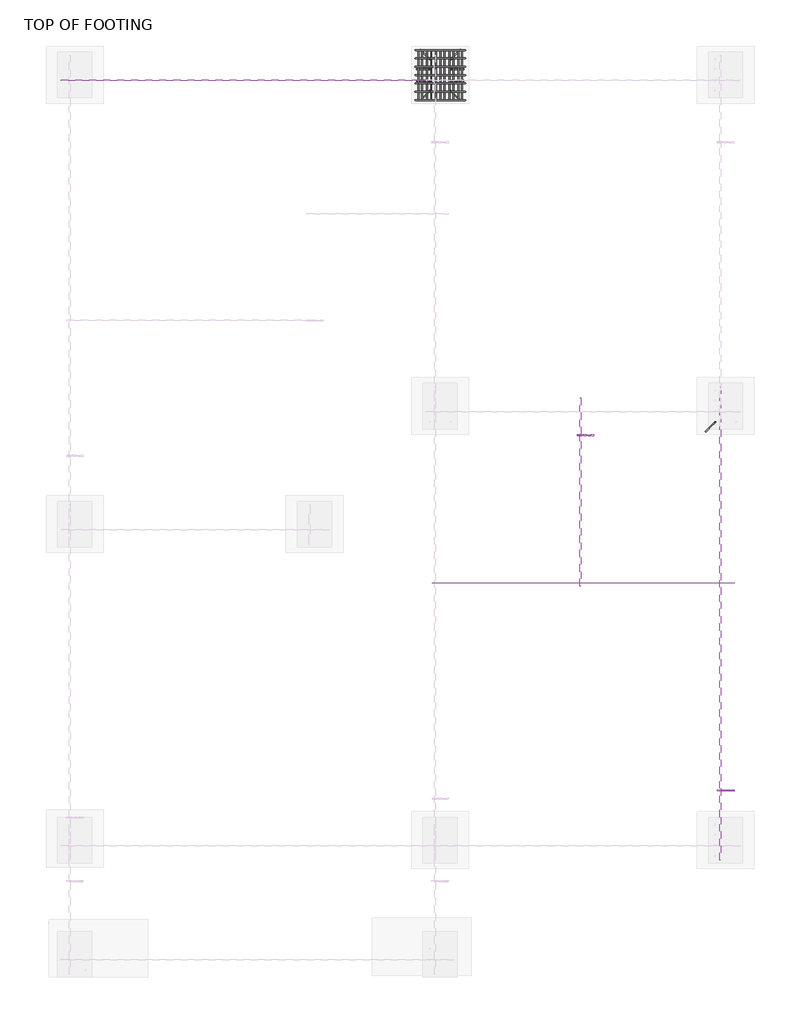
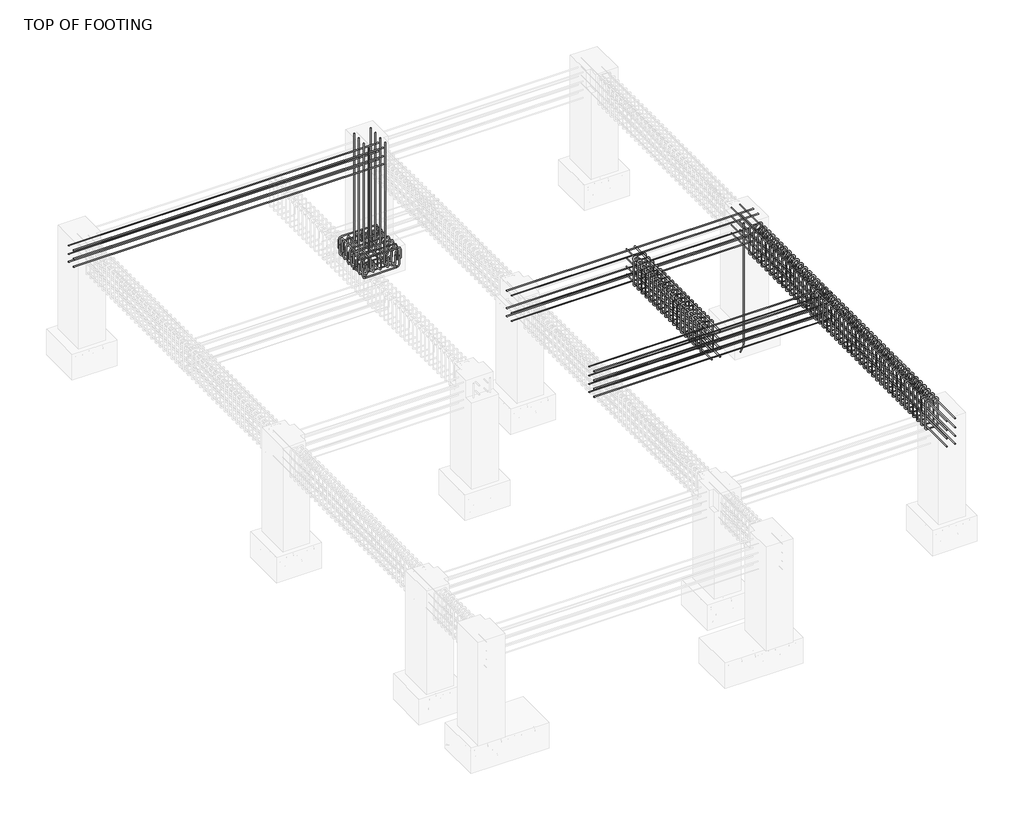
# One storey, part 7 of 8: 31 reinforcing bars.
"""IFC4 building model written with IfcOpenShell, lengths in millimetres."""

from ifc_helpers import new_model, si_unit, point, frame, origin, place, context, project, spatial, polyline, circle_curve, trimmed, segment, composite_curve, source, transform, mapped, element, save
from ifc_brep_helpers import swept_disk

model = new_model("IFC4")

# Units and contexts
model_context = context("Model", 3, world=origin())
ifc_project = project(units=[si_unit("LENGTHUNIT", "METRE", prefix="MILLI")], contexts=[model_context])

# Site, building, storey
site = spatial("IfcSite", under=ifc_project)
building = spatial("IfcBuilding", under=site)
storey = spatial("IfcBuildingStorey", under=building, Name="TOP OF FOOTING", Elevation=-1828.8)

# Reinforcing bars
placement = place(None, origin())
reinforcing_bar_shape = source(origin(), model_context, "Body", "SolidModel", [
    swept_disk(composite_curve([segment(polyline([(-1395.5877818, 9895.6420243, -2021.245224), (-1395.5877818, 9895.6420243, -2168.545224)]), True, "CONTINUOUS"), segment(trimmed(circle_curve(frame((-1441.9377818, 9895.6420243, -2168.545224), z_axis=(0.0, 1.0, 0.0), x_axis=(46.350000000000136, 0.0, 0.0)), 46.35), [point((-1395.5877818, 9895.6420243, -2168.545224))], [point((-1441.9377818, 9895.6420243, -2214.895224))], True, "CARTESIAN"), True, "CONTINUOUS"), segment(polyline([(-1441.9377818, 9895.6420243, -2214.895224), (-1962.8758647, 9895.6420243, -2214.895224)]), True, "CONTINUOUS"), segment(trimmed(circle_curve(frame((-1962.8758647, 9895.6420243, -2168.545224), z_axis=(0.0, 1.0, 0.0), x_axis=(0.0, 0.0, -46.34999999999991)), 46.35), [point((-1962.8758647, 9895.6420243, -2214.895224))], [point((-2009.2258647, 9895.6420243, -2168.545224))], True, "CARTESIAN"), True, "CONTINUOUS"), segment(polyline([(-2009.2258647, 9895.6420243, -2168.545224), (-2009.2258647, 9895.6420243, -2021.245224)]), True, "CONTINUOUS")], self_intersect=False), 6.35),
])
element("IfcReinforcingBar", 1, at=placement, inside=storey, context=model_context, shape_type="MappedRepresentation", body=[
    mapped(reinforcing_bar_shape, transform((0.0, 0.0, 0.0), x_axis=(1.0, 0.0, 0.0), y_axis=(0.0, 1.0, 0.0), z_axis=(0.0, 0.0, 1.0))),
    mapped(reinforcing_bar_shape, transform((0.0, -109.55, 0.0), x_axis=(1.0, 0.0, 0.0), y_axis=(0.0, 1.0, 0.0), z_axis=(0.0, 0.0, 1.0))),
    mapped(reinforcing_bar_shape, transform((0.0, -219.1, 0.0), x_axis=(1.0, 0.0, 0.0), y_axis=(0.0, 1.0, 0.0), z_axis=(0.0, 0.0, 1.0))),
    mapped(reinforcing_bar_shape, transform((0.0, -328.65, 0.0), x_axis=(1.0, 0.0, 0.0), y_axis=(0.0, 1.0, 0.0), z_axis=(0.0, 0.0, 1.0))),
    mapped(reinforcing_bar_shape, transform((0.0, -438.2, 0.0), x_axis=(1.0, 0.0, 0.0), y_axis=(0.0, 1.0, 0.0), z_axis=(0.0, 0.0, 1.0))),
    mapped(reinforcing_bar_shape, transform((0.0, -547.75, 0.0), x_axis=(1.0, 0.0, 0.0), y_axis=(0.0, 1.0, 0.0), z_axis=(0.0, 0.0, 1.0))),
    mapped(reinforcing_bar_shape, transform((0.0, -657.3, 0.0), x_axis=(1.0, 0.0, 0.0), y_axis=(0.0, 1.0, 0.0), z_axis=(0.0, 0.0, 1.0))),
])
reinforcing_bar_2_shape = source(origin(), model_context, "Body", "SolidModel", [
    swept_disk(composite_curve([segment(polyline([(-2031.1461367, 9895.6420243, -2068.8), (-2031.1461367, 9895.6420243, -1921.5)]), True, "CONTINUOUS"), segment(trimmed(circle_curve(frame((-1984.7961367, 9895.6420243, -1921.5), z_axis=(0.0, 1.0, 0.0), x_axis=(-46.34999999999991, 0.0, 0.0)), 46.35), [point((-2031.1461367, 9895.6420243, -1921.5))], [point((-1984.7961367, 9895.6420243, -1875.15))], True, "CARTESIAN"), True, "CONTINUOUS"), segment(polyline([(-1984.7961367, 9895.6420243, -1875.15), (-1420.1961367, 9895.6420243, -1875.15)]), True, "CONTINUOUS"), segment(trimmed(circle_curve(frame((-1420.1961367, 9895.6420243, -1921.5), z_axis=(0.0, 1.0, 0.0), x_axis=(0.0, 0.0, 46.34999999999991)), 46.35), [point((-1420.1961367, 9895.6420243, -1875.15))], [point((-1373.8461367, 9895.6420243, -1921.5))], True, "CARTESIAN"), True, "CONTINUOUS"), segment(polyline([(-1373.8461367, 9895.6420243, -1921.5), (-1373.8461367, 9895.6420243, -2068.8)]), True, "CONTINUOUS")], self_intersect=False), 6.35),
])
element("IfcReinforcingBar", 2, at=placement, inside=storey, context=model_context, shape_type="MappedRepresentation", body=[
    mapped(reinforcing_bar_2_shape, transform((0.0, 0.0, 0.0), x_axis=(1.0, 0.0, 0.0), y_axis=(0.0, 1.0, 0.0), z_axis=(0.0, 0.0, 1.0))),
    mapped(reinforcing_bar_2_shape, transform((0.0, -109.55, 0.0), x_axis=(1.0, 0.0, 0.0), y_axis=(0.0, 1.0, 0.0), z_axis=(0.0, 0.0, 1.0))),
    mapped(reinforcing_bar_2_shape, transform((0.0, -219.1, 0.0), x_axis=(1.0, 0.0, 0.0), y_axis=(0.0, 1.0, 0.0), z_axis=(0.0, 0.0, 1.0))),
    mapped(reinforcing_bar_2_shape, transform((0.0, -328.65, 0.0), x_axis=(1.0, 0.0, 0.0), y_axis=(0.0, 1.0, 0.0), z_axis=(0.0, 0.0, 1.0))),
    mapped(reinforcing_bar_2_shape, transform((0.0, -438.2, 0.0), x_axis=(1.0, 0.0, 0.0), y_axis=(0.0, 1.0, 0.0), z_axis=(0.0, 0.0, 1.0))),
    mapped(reinforcing_bar_2_shape, transform((0.0, -547.75, 0.0), x_axis=(1.0, 0.0, 0.0), y_axis=(0.0, 1.0, 0.0), z_axis=(0.0, 0.0, 1.0))),
    mapped(reinforcing_bar_2_shape, transform((0.0, -657.3, 0.0), x_axis=(1.0, 0.0, 0.0), y_axis=(0.0, 1.0, 0.0), z_axis=(0.0, 0.0, 1.0))),
])
reinforcing_bar_3_shape = source(origin(), model_context, "Body", "SolidModel", [
    swept_disk(composite_curve([segment(polyline([(-1419.0253093, 9895.6420243, -2080.9203068), (-1419.0253093, 9895.6420243, -1933.6203068)]), True, "CONTINUOUS"), segment(trimmed(circle_curve(frame((-1419.0253093, 9849.2920243, -1933.6203068), z_axis=(1.0, 0.0, 0.0), x_axis=(0.0, 46.349999999998545, 0.0)), 46.35), [point((-1419.0253093, 9895.6420243, -1933.6203068))], [point((-1419.0253093, 9849.2920243, -1887.2703068))], True, "CARTESIAN"), True, "CONTINUOUS"), segment(polyline([(-1419.0253093, 9849.2920243, -1887.2703068), (-1419.0253093, 9284.6920243, -1887.2703068)]), True, "CONTINUOUS"), segment(trimmed(circle_curve(frame((-1419.0253093, 9284.6920243, -1933.6203068), z_axis=(1.0, 0.0, 0.0), x_axis=(0.0, 0.0, 46.34999999999991)), 46.35), [point((-1419.0253093, 9284.6920243, -1887.2703068))], [point((-1419.0253093, 9238.3420243, -1933.6203068))], True, "CARTESIAN"), True, "CONTINUOUS"), segment(polyline([(-1419.0253093, 9238.3420243, -1933.6203068), (-1419.0253093, 9238.3420243, -2080.9203068)]), True, "CONTINUOUS")], self_intersect=False), 6.35),
])
element("IfcReinforcingBar", 3, at=placement, inside=storey, context=model_context, shape_type="MappedRepresentation", body=[
    mapped(reinforcing_bar_3_shape, transform((0.0, 0.0, 0.0), x_axis=(1.0, 0.0, 0.0), y_axis=(0.0, 1.0, 0.0), z_axis=(0.0, 0.0, 1.0))),
    mapped(reinforcing_bar_3_shape, transform((-113.9683653, 0.0, 0.0), x_axis=(1.0, 0.0, 0.0), y_axis=(0.0, 1.0, 0.0), z_axis=(0.0, 0.0, 1.0))),
    mapped(reinforcing_bar_3_shape, transform((-227.9367307, 0.0, 0.0), x_axis=(1.0, 0.0, 0.0), y_axis=(0.0, 1.0, 0.0), z_axis=(0.0, 0.0, 1.0))),
    mapped(reinforcing_bar_3_shape, transform((-341.905096, 0.0, 0.0), x_axis=(1.0, 0.0, 0.0), y_axis=(0.0, 1.0, 0.0), z_axis=(0.0, 0.0, 1.0))),
    mapped(reinforcing_bar_3_shape, transform((-455.8734613, 0.0, 0.0), x_axis=(1.0, 0.0, 0.0), y_axis=(0.0, 1.0, 0.0), z_axis=(0.0, 0.0, 1.0))),
    mapped(reinforcing_bar_3_shape, transform((-569.8418267, 0.0, 0.0), x_axis=(1.0, 0.0, 0.0), y_axis=(0.0, 1.0, 0.0), z_axis=(0.0, 0.0, 1.0))),
])
reinforcing_bar_4_shape = source(origin(), model_context, "Body", "SolidModel", [
    swept_disk(composite_curve([segment(polyline([(-1941.3656272, 9895.6420243, -1984.9681267), (-1941.3656272, 9895.6420243, -2132.2681267)]), True, "CONTINUOUS"), segment(trimmed(circle_curve(frame((-1941.3656272, 9849.2920243, -2132.2681267), z_axis=(-1.0, 0.0, 0.0), x_axis=(0.0, 46.349999999998545, 0.0)), 46.35), [point((-1941.3656272, 9895.6420243, -2132.2681267))], [point((-1941.3656272, 9849.2920243, -2178.6181267))], True, "CARTESIAN"), True, "CONTINUOUS"), segment(polyline([(-1941.3656272, 9849.2920243, -2178.6181267), (-1941.3656272, 9284.6920243, -2178.6181267)]), True, "CONTINUOUS"), segment(trimmed(circle_curve(frame((-1941.3656272, 9284.6920243, -2132.2681267), z_axis=(-1.0, 0.0, 0.0), x_axis=(0.0, 0.0, -46.350000000000364)), 46.35), [point((-1941.3656272, 9284.6920243, -2178.6181267))], [point((-1941.3656272, 9238.3420243, -2132.2681267))], True, "CARTESIAN"), True, "CONTINUOUS"), segment(polyline([(-1941.3656272, 9238.3420243, -2132.2681267), (-1941.3656272, 9238.3420243, -1984.9681267)]), True, "CONTINUOUS")], self_intersect=False), 6.35),
])
element("IfcReinforcingBar", 4, at=placement, inside=storey, context=model_context, shape_type="MappedRepresentation", body=[
    mapped(reinforcing_bar_4_shape, transform((0.0, 0.0, 0.0), x_axis=(1.0, 0.0, 0.0), y_axis=(0.0, 1.0, 0.0), z_axis=(0.0, 0.0, 1.0))),
    mapped(reinforcing_bar_4_shape, transform((119.2770606, 0.0, 0.0), x_axis=(1.0, 0.0, 0.0), y_axis=(0.0, 1.0, 0.0), z_axis=(0.0, 0.0, 1.0))),
    mapped(reinforcing_bar_4_shape, transform((238.5541211, 0.0, 0.0), x_axis=(1.0, 0.0, 0.0), y_axis=(0.0, 1.0, 0.0), z_axis=(0.0, 0.0, 1.0))),
    mapped(reinforcing_bar_4_shape, transform((357.8311817, 0.0, 0.0), x_axis=(1.0, 0.0, 0.0), y_axis=(0.0, 1.0, 0.0), z_axis=(0.0, 0.0, 1.0))),
    mapped(reinforcing_bar_4_shape, transform((477.1082423, 0.0, 0.0), x_axis=(1.0, 0.0, 0.0), y_axis=(0.0, 1.0, 0.0), z_axis=(0.0, 0.0, 1.0))),
])
reinforcing_bar_5_shape = source(origin(), model_context, "Body", "SolidModel", [
    swept_disk(composite_curve([segment(polyline([(-2015.4438347, 9642.1344308, -2192.6897268), (-1887.1151723, 9642.1344308, -2192.6897268)]), True, "CONTINUOUS"), segment(trimmed(circle_curve(frame((-1887.1151723, 9642.1344308, -2146.3397268), z_axis=(0.0, -1.0, 0.0), x_axis=(0.0, 0.0, -46.34999999999991)), 46.35), [point((-1887.1151723, 9642.1344308, -2192.6897268))], [point((-1840.7651723, 9642.1344308, -2146.3397268))], True, "CARTESIAN"), True, "CONTINUOUS"), segment(polyline([(-1840.7651723, 9642.1344308, -2146.3397268), (-1840.7651723, 9642.1344308, -40.0)]), True, "CONTINUOUS")], self_intersect=False), 6.35),
])
element("IfcReinforcingBar", 5, at=placement, inside=storey, context=model_context, shape_type="MappedRepresentation", body=[
    mapped(reinforcing_bar_5_shape, transform((0.0, 0.0, 0.0), x_axis=(1.0, 0.0, 0.0), y_axis=(0.0, 1.0, 0.0), z_axis=(0.0, 0.0, 1.0))),
    mapped(reinforcing_bar_5_shape, transform((0.0, -147.7903727, 0.0), x_axis=(1.0, 0.0, 0.0), y_axis=(0.0, 1.0, 0.0), z_axis=(0.0, 0.0, 1.0))),
])
element("IfcReinforcingBar", 6, at=placement, inside=storey, context=model_context, shape_type="SolidModel", body=[
    swept_disk(composite_curve([segment(polyline([(-1968.0144002, 9232.6300935, -2192.6897268), (-1873.5395717, 9327.1049221, -2192.6897268)]), True, "CONTINUOUS"), segment(trimmed(circle_curve(frame((-1873.5395717, 9327.1049221, -2146.3397268), z_axis=(0.7071067811865476, -0.7071067811865475, 0.0), x_axis=(0.0, 0.0, -46.34999999999991)), 46.35), [point((-1873.5395717, 9327.1049221, -2192.6897268))], [point((-1840.7651723, 9359.8793214, -2146.3397268))], True, "CARTESIAN"), True, "CONTINUOUS"), segment(polyline([(-1840.7651723, 9359.8793214, -2146.3397268), (-1840.7651723, 9359.8793214, -40.0)]), True, "CONTINUOUS")], self_intersect=False), 6.35),
])
element("IfcReinforcingBar", 7, at=placement, inside=storey, context=model_context, shape_type="SolidModel", body=[
    swept_disk(composite_curve([segment(polyline([(-1436.9778732, 9232.6300935, -2192.6897268), (-1531.4527018, 9327.1049221, -2192.6897268)]), True, "CONTINUOUS"), segment(trimmed(circle_curve(frame((-1531.4527018, 9327.1049221, -2146.3397268), z_axis=(0.7071067811865753, 0.7071067811865197, 0.0), x_axis=(0.0, 0.0, -46.34999999999991)), 46.35), [point((-1531.4527018, 9327.1049221, -2192.6897268))], [point((-1564.2271011, 9359.8793214, -2146.3397268))], True, "CARTESIAN"), True, "CONTINUOUS"), segment(polyline([(-1564.2271011, 9359.8793214, -2146.3397268), (-1564.2271011, 9359.8793214, -40.0)]), True, "CONTINUOUS")], self_intersect=False), 6.35),
])
element("IfcReinforcingBar", 8, at=placement, inside=storey, context=model_context, shape_type="SolidModel", body=[
    swept_disk(composite_curve([segment(polyline([(-1968.0144002, 9901.353955, -2192.6897268), (-1873.5395717, 9806.8791264, -2192.6897268)]), True, "CONTINUOUS"), segment(trimmed(circle_curve(frame((-1873.5395717, 9806.8791264, -2146.3397268), z_axis=(-0.7071067811865389, -0.7071067811865561, 0.0), x_axis=(0.0, 0.0, -46.34999999999991)), 46.35), [point((-1873.5395717, 9806.8791264, -2192.6897268))], [point((-1840.7651723, 9774.1047271, -2146.3397268))], True, "CARTESIAN"), True, "CONTINUOUS"), segment(polyline([(-1840.7651723, 9774.1047271, -2146.3397268), (-1840.7651723, 9774.1047271, -40.0)]), True, "CONTINUOUS")], self_intersect=False), 6.35),
])
element("IfcReinforcingBar", 9, at=placement, inside=storey, context=model_context, shape_type="SolidModel", body=[
    swept_disk(composite_curve([segment(polyline([(-1436.9778732, 9901.353955, -2192.6897268), (-1531.4527018, 9806.8791264, -2192.6897268)]), True, "CONTINUOUS"), segment(trimmed(circle_curve(frame((-1531.4527018, 9806.8791264, -2146.3397268), z_axis=(-0.707106781186584, 0.707106781186511, 0.0), x_axis=(0.0, 0.0, -46.34999999999991)), 46.35), [point((-1531.4527018, 9806.8791264, -2192.6897268))], [point((-1564.2271011, 9774.1047271, -2146.3397268))], True, "CARTESIAN"), True, "CONTINUOUS"), segment(polyline([(-1564.2271011, 9774.1047271, -2146.3397268), (-1564.2271011, 9774.1047271, -40.0)]), True, "CONTINUOUS")], self_intersect=False), 6.35),
])
reinforcing_bar_6_shape = source(origin(), model_context, "Body", "SolidModel", [
    swept_disk(composite_curve([segment(polyline([(-1389.5484388, 9642.1344308, -2192.6897268), (-1517.8771011, 9642.1344308, -2192.6897268)]), True, "CONTINUOUS"), segment(trimmed(circle_curve(frame((-1517.8771011, 9642.1344308, -2146.3397268), z_axis=(0.0, 1.0, 0.0), x_axis=(0.0, 0.0, -46.34999999999991)), 46.35), [point((-1517.8771011, 9642.1344308, -2192.6897268))], [point((-1564.2271011, 9642.1344308, -2146.3397268))], True, "CARTESIAN"), True, "CONTINUOUS"), segment(polyline([(-1564.2271011, 9642.1344308, -2146.3397268), (-1564.2271011, 9642.1344308, -40.0)]), True, "CONTINUOUS")], self_intersect=False), 6.35),
])
element("IfcReinforcingBar", 10, at=placement, inside=storey, context=model_context, shape_type="MappedRepresentation", body=[
    mapped(reinforcing_bar_6_shape, transform((0.0, 0.0, 0.0), x_axis=(1.0, 0.0, 0.0), y_axis=(0.0, 1.0, 0.0), z_axis=(0.0, 0.0, 1.0))),
    mapped(reinforcing_bar_6_shape, transform((0.0, -147.7903727, 0.0), x_axis=(1.0, 0.0, 0.0), y_axis=(0.0, 1.0, 0.0), z_axis=(0.0, 0.0, 1.0))),
])
element("IfcReinforcingBar", 11, at=placement, inside=storey, context=model_context, shape_type="SolidModel", body=[
    swept_disk(composite_curve([segment(polyline([(1781.9855998, 4882.6300935, -2192.6897268), (1876.4604283, 4977.1049221, -2192.6897268)]), True, "CONTINUOUS"), segment(trimmed(circle_curve(frame((1876.4604283, 4977.1049221, -2146.3397268), z_axis=(0.7071067811865476, -0.7071067811865475, 0.0), x_axis=(0.0, 0.0, -46.34999999999991)), 46.35), [point((1876.4604283, 4977.1049221, -2192.6897268))], [point((1909.2348277, 5009.8793214, -2146.3397268))], True, "CARTESIAN"), True, "CONTINUOUS"), segment(polyline([(1909.2348277, 5009.8793214, -2146.3397268), (1909.2348277, 5009.8793214, -40.0)]), True, "CONTINUOUS")], self_intersect=False), 6.35),
])
reinforcing_bar_7_shape = source(origin(), model_context, "Body", "SolidModel", [
    swept_disk(composite_curve([segment(polyline([(-6687.4961367, 9636.6137956, -522.7), (-1517.4961367, 9636.6137956, -522.7)]), True, "CONTINUOUS")], self_intersect=False), 6.35),
])
element("IfcReinforcingBar", 12, at=placement, inside=storey, context=model_context, shape_type="MappedRepresentation", body=[
    mapped(reinforcing_bar_7_shape, transform((0.0, 0.0, 0.0), x_axis=(1.0, 0.0, 0.0), y_axis=(0.0, 1.0, 0.0), z_axis=(0.0, 0.0, 1.0))),
    mapped(reinforcing_bar_7_shape, transform((0.0, -139.7429418, 0.0), x_axis=(1.0, 0.0, 0.0), y_axis=(0.0, 1.0, 0.0), z_axis=(0.0, 0.0, 1.0))),
])
reinforcing_bar_8_shape = source(origin(), model_context, "Body", "SolidModel", [
    swept_disk(composite_curve([segment(polyline([(-6687.4961367, 9636.6137956, -382.7), (-1517.4961367, 9636.6137956, -382.7)]), True, "CONTINUOUS")], self_intersect=False), 6.35),
])
element("IfcReinforcingBar", 13, at=placement, inside=storey, context=model_context, shape_type="MappedRepresentation", body=[
    mapped(reinforcing_bar_8_shape, transform((0.0, 0.0, 0.0), x_axis=(1.0, 0.0, 0.0), y_axis=(0.0, 1.0, 0.0), z_axis=(0.0, 0.0, 1.0))),
    mapped(reinforcing_bar_8_shape, transform((0.0, -139.7429418, 0.0), x_axis=(1.0, 0.0, 0.0), y_axis=(0.0, 1.0, 0.0), z_axis=(0.0, 0.0, 1.0))),
])
reinforcing_bar_9_shape = source(origin(), model_context, "Body", "SolidModel", [
    swept_disk(composite_curve([segment(polyline([(-6687.4961367, 9636.6137956, -232.7), (-1517.4961367, 9636.6137956, -232.7)]), True, "CONTINUOUS")], self_intersect=False), 6.35),
])
element("IfcReinforcingBar", 14, at=placement, inside=storey, context=model_context, shape_type="MappedRepresentation", body=[
    mapped(reinforcing_bar_9_shape, transform((0.0, 0.0, 0.0), x_axis=(1.0, 0.0, 0.0), y_axis=(0.0, 1.0, 0.0), z_axis=(0.0, 0.0, 1.0))),
    mapped(reinforcing_bar_9_shape, transform((0.0, -139.7429418, 0.0), x_axis=(1.0, 0.0, 0.0), y_axis=(0.0, 1.0, 0.0), z_axis=(0.0, 0.0, 1.0))),
])
reinforcing_bar_10_shape = source(origin(), model_context, "Body", "SolidModel", [
    swept_disk(composite_curve([segment(polyline([(2041.8925027, -176.6579757, -111.2757654), (2097.6360657, -176.6579757, -55.5322024)]), True, "CONTINUOUS"), segment(trimmed(circle_curve(frame((2119.8038633, -176.6579757, -77.7), z_axis=(0.0, 1.0, 0.0), x_axis=(-22.167797600000085, 0.0, 22.1677976)), 31.35), [point((2097.6360657, -176.6579757, -55.5322024))], [point((2151.1538633, -176.6579757, -77.7))], True, "CARTESIAN"), True, "CONTINUOUS"), segment(polyline([(2151.1538633, -176.6579757, -77.7), (2151.1538633, -176.6579757, -522.3)]), True, "CONTINUOUS"), segment(trimmed(circle_curve(frame((2119.8038633, -176.6579757, -522.3), z_axis=(0.0, 1.0, 0.0), x_axis=(31.34999999999991, 0.0, 0.0)), 31.35), [point((2151.1538633, -176.6579757, -522.3))], [point((2119.8038633, -176.6579757, -553.65))], True, "CARTESIAN"), True, "CONTINUOUS"), segment(polyline([(2119.8038633, -176.6579757, -553.65), (1975.2038633, -176.6579757, -553.65)]), True, "CONTINUOUS"), segment(trimmed(circle_curve(frame((1975.2038633, -177.4425614, -522.3098193), z_axis=(0.0, 0.9996867842138424, 0.025026655153786322), x_axis=(0.0, 0.7845856999999796, -31.34018070000002)), 31.35), [point((1975.2038633, -176.6579757, -553.65))], [point((1943.8538633, -177.4425614, -522.3098193))], True, "CARTESIAN"), True, "CONTINUOUS"), segment(polyline([(1943.8538633, -177.4425614, -522.3098193), (1943.8538633, -188.5733901, -77.6901807)]), True, "CONTINUOUS"), segment(trimmed(circle_curve(frame((1975.2038633, -188.5733901, -77.6901807), z_axis=(0.0, 0.9996867842138424, 0.025026655153786322), x_axis=(-31.34999999999991, 0.0, 0.0)), 31.35), [point((1943.8538633, -188.5733901, -77.6901807))], [point((1975.2038633, -189.3579757, -46.35))], True, "CARTESIAN"), True, "CONTINUOUS"), segment(polyline([(1975.2038633, -189.3579757, -46.35), (2119.8038633, -189.3579757, -46.35)]), True, "CONTINUOUS"), segment(trimmed(circle_curve(frame((2119.8038633, -189.3579757, -77.7), z_axis=(0.0, 1.0, 0.0), x_axis=(0.0, 0.0, 31.35)), 31.35), [point((2119.8038633, -189.3579757, -46.35))], [point((2141.9716609, -189.3579757, -99.8677976))], True, "CARTESIAN"), True, "CONTINUOUS"), segment(polyline([(2141.9716609, -189.3579757, -99.8677976), (2086.2280979, -189.3579757, -155.6113605)]), True, "CONTINUOUS")], self_intersect=False), 6.35),
])
element("IfcReinforcingBar", 15, at=placement, inside=storey, context=model_context, shape_type="MappedRepresentation", body=[
    mapped(reinforcing_bar_10_shape, transform((0.0, 0.0, 0.0), x_axis=(1.0, 0.0, 0.0), y_axis=(0.0, 1.0, 0.0), z_axis=(0.0, 0.0, 1.0))),
    mapped(reinforcing_bar_10_shape, transform((0.0, 118.3093023, 0.0), x_axis=(1.0, 0.0, 0.0), y_axis=(0.0, 1.0, 0.0), z_axis=(0.0, 0.0, 1.0))),
    mapped(reinforcing_bar_10_shape, transform((0.0, 236.6186047, 0.0), x_axis=(1.0, 0.0, 0.0), y_axis=(0.0, 1.0, 0.0), z_axis=(0.0, 0.0, 1.0))),
    mapped(reinforcing_bar_10_shape, transform((0.0, 354.927907, 0.0), x_axis=(1.0, 0.0, 0.0), y_axis=(0.0, 1.0, 0.0), z_axis=(0.0, 0.0, 1.0))),
    mapped(reinforcing_bar_10_shape, transform((0.0, 473.2372093, 0.0), x_axis=(1.0, 0.0, 0.0), y_axis=(0.0, 1.0, 0.0), z_axis=(0.0, 0.0, 1.0))),
    mapped(reinforcing_bar_10_shape, transform((0.0, 591.5465116, 0.0), x_axis=(1.0, 0.0, 0.0), y_axis=(0.0, 1.0, 0.0), z_axis=(0.0, 0.0, 1.0))),
    mapped(reinforcing_bar_10_shape, transform((0.0, 709.855814, 0.0), x_axis=(1.0, 0.0, 0.0), y_axis=(0.0, 1.0, 0.0), z_axis=(0.0, 0.0, 1.0))),
    mapped(reinforcing_bar_10_shape, transform((0.0, 828.1651163, 0.0), x_axis=(1.0, 0.0, 0.0), y_axis=(0.0, 1.0, 0.0), z_axis=(0.0, 0.0, 1.0))),
    mapped(reinforcing_bar_10_shape, transform((0.0, 946.4744186, 0.0), x_axis=(1.0, 0.0, 0.0), y_axis=(0.0, 1.0, 0.0), z_axis=(0.0, 0.0, 1.0))),
    mapped(reinforcing_bar_10_shape, transform((0.0, 1064.7837209, 0.0), x_axis=(1.0, 0.0, 0.0), y_axis=(0.0, 1.0, 0.0), z_axis=(0.0, 0.0, 1.0))),
    mapped(reinforcing_bar_10_shape, transform((0.0, 1183.0930233, 0.0), x_axis=(1.0, 0.0, 0.0), y_axis=(0.0, 1.0, 0.0), z_axis=(0.0, 0.0, 1.0))),
    mapped(reinforcing_bar_10_shape, transform((0.0, 1301.4023256, 0.0), x_axis=(1.0, 0.0, 0.0), y_axis=(0.0, 1.0, 0.0), z_axis=(0.0, 0.0, 1.0))),
    mapped(reinforcing_bar_10_shape, transform((0.0, 1419.7116279, 0.0), x_axis=(1.0, 0.0, 0.0), y_axis=(0.0, 1.0, 0.0), z_axis=(0.0, 0.0, 1.0))),
    mapped(reinforcing_bar_10_shape, transform((0.0, 1538.0209302, 0.0), x_axis=(1.0, 0.0, 0.0), y_axis=(0.0, 1.0, 0.0), z_axis=(0.0, 0.0, 1.0))),
    mapped(reinforcing_bar_10_shape, transform((0.0, 1656.3302326, 0.0), x_axis=(1.0, 0.0, 0.0), y_axis=(0.0, 1.0, 0.0), z_axis=(0.0, 0.0, 1.0))),
    mapped(reinforcing_bar_10_shape, transform((0.0, 1774.6395349, 0.0), x_axis=(1.0, 0.0, 0.0), y_axis=(0.0, 1.0, 0.0), z_axis=(0.0, 0.0, 1.0))),
    mapped(reinforcing_bar_10_shape, transform((0.0, 1892.9488372, 0.0), x_axis=(1.0, 0.0, 0.0), y_axis=(0.0, 1.0, 0.0), z_axis=(0.0, 0.0, 1.0))),
    mapped(reinforcing_bar_10_shape, transform((0.0, 2011.2581395, 0.0), x_axis=(1.0, 0.0, 0.0), y_axis=(0.0, 1.0, 0.0), z_axis=(0.0, 0.0, 1.0))),
    mapped(reinforcing_bar_10_shape, transform((0.0, 2129.5674419, 0.0), x_axis=(1.0, 0.0, 0.0), y_axis=(0.0, 1.0, 0.0), z_axis=(0.0, 0.0, 1.0))),
    mapped(reinforcing_bar_10_shape, transform((0.0, 2247.8767442, 0.0), x_axis=(1.0, 0.0, 0.0), y_axis=(0.0, 1.0, 0.0), z_axis=(0.0, 0.0, 1.0))),
    mapped(reinforcing_bar_10_shape, transform((0.0, 2366.1860465, 0.0), x_axis=(1.0, 0.0, 0.0), y_axis=(0.0, 1.0, 0.0), z_axis=(0.0, 0.0, 1.0))),
    mapped(reinforcing_bar_10_shape, transform((0.0, 2484.4953488, 0.0), x_axis=(1.0, 0.0, 0.0), y_axis=(0.0, 1.0, 0.0), z_axis=(0.0, 0.0, 1.0))),
    mapped(reinforcing_bar_10_shape, transform((0.0, 2602.8046512, 0.0), x_axis=(1.0, 0.0, 0.0), y_axis=(0.0, 1.0, 0.0), z_axis=(0.0, 0.0, 1.0))),
    mapped(reinforcing_bar_10_shape, transform((0.0, 2721.1139535, 0.0), x_axis=(1.0, 0.0, 0.0), y_axis=(0.0, 1.0, 0.0), z_axis=(0.0, 0.0, 1.0))),
    mapped(reinforcing_bar_10_shape, transform((0.0, 2839.4232558, 0.0), x_axis=(1.0, 0.0, 0.0), y_axis=(0.0, 1.0, 0.0), z_axis=(0.0, 0.0, 1.0))),
    mapped(reinforcing_bar_10_shape, transform((0.0, 2957.7325581, 0.0), x_axis=(1.0, 0.0, 0.0), y_axis=(0.0, 1.0, 0.0), z_axis=(0.0, 0.0, 1.0))),
    mapped(reinforcing_bar_10_shape, transform((0.0, 3076.0418605, 0.0), x_axis=(1.0, 0.0, 0.0), y_axis=(0.0, 1.0, 0.0), z_axis=(0.0, 0.0, 1.0))),
    mapped(reinforcing_bar_10_shape, transform((0.0, 3194.3511628, 0.0), x_axis=(1.0, 0.0, 0.0), y_axis=(0.0, 1.0, 0.0), z_axis=(0.0, 0.0, 1.0))),
    mapped(reinforcing_bar_10_shape, transform((0.0, 3312.6604651, 0.0), x_axis=(1.0, 0.0, 0.0), y_axis=(0.0, 1.0, 0.0), z_axis=(0.0, 0.0, 1.0))),
    mapped(reinforcing_bar_10_shape, transform((0.0, 3430.9697674, 0.0), x_axis=(1.0, 0.0, 0.0), y_axis=(0.0, 1.0, 0.0), z_axis=(0.0, 0.0, 1.0))),
    mapped(reinforcing_bar_10_shape, transform((0.0, 3549.2790698, 0.0), x_axis=(1.0, 0.0, 0.0), y_axis=(0.0, 1.0, 0.0), z_axis=(0.0, 0.0, 1.0))),
    mapped(reinforcing_bar_10_shape, transform((0.0, 3667.5883721, 0.0), x_axis=(1.0, 0.0, 0.0), y_axis=(0.0, 1.0, 0.0), z_axis=(0.0, 0.0, 1.0))),
    mapped(reinforcing_bar_10_shape, transform((0.0, 3785.8976744, 0.0), x_axis=(1.0, 0.0, 0.0), y_axis=(0.0, 1.0, 0.0), z_axis=(0.0, 0.0, 1.0))),
    mapped(reinforcing_bar_10_shape, transform((0.0, 3904.2069767, 0.0), x_axis=(1.0, 0.0, 0.0), y_axis=(0.0, 1.0, 0.0), z_axis=(0.0, 0.0, 1.0))),
    mapped(reinforcing_bar_10_shape, transform((0.0, 4022.5162791, 0.0), x_axis=(1.0, 0.0, 0.0), y_axis=(0.0, 1.0, 0.0), z_axis=(0.0, 0.0, 1.0))),
    mapped(reinforcing_bar_10_shape, transform((0.0, 4140.8255814, 0.0), x_axis=(1.0, 0.0, 0.0), y_axis=(0.0, 1.0, 0.0), z_axis=(0.0, 0.0, 1.0))),
    mapped(reinforcing_bar_10_shape, transform((0.0, 4259.1348837, 0.0), x_axis=(1.0, 0.0, 0.0), y_axis=(0.0, 1.0, 0.0), z_axis=(0.0, 0.0, 1.0))),
    mapped(reinforcing_bar_10_shape, transform((0.0, 4377.444186, 0.0), x_axis=(1.0, 0.0, 0.0), y_axis=(0.0, 1.0, 0.0), z_axis=(0.0, 0.0, 1.0))),
    mapped(reinforcing_bar_10_shape, transform((0.0, 4495.7534884, 0.0), x_axis=(1.0, 0.0, 0.0), y_axis=(0.0, 1.0, 0.0), z_axis=(0.0, 0.0, 1.0))),
    mapped(reinforcing_bar_10_shape, transform((0.0, 4614.0627907, 0.0), x_axis=(1.0, 0.0, 0.0), y_axis=(0.0, 1.0, 0.0), z_axis=(0.0, 0.0, 1.0))),
    mapped(reinforcing_bar_10_shape, transform((0.0, 4732.372093, 0.0), x_axis=(1.0, 0.0, 0.0), y_axis=(0.0, 1.0, 0.0), z_axis=(0.0, 0.0, 1.0))),
    mapped(reinforcing_bar_10_shape, transform((0.0, 4850.6813953, 0.0), x_axis=(1.0, 0.0, 0.0), y_axis=(0.0, 1.0, 0.0), z_axis=(0.0, 0.0, 1.0))),
    mapped(reinforcing_bar_10_shape, transform((0.0, 4968.9906977, 0.0), x_axis=(1.0, 0.0, 0.0), y_axis=(0.0, 1.0, 0.0), z_axis=(0.0, 0.0, 1.0))),
    mapped(reinforcing_bar_10_shape, transform((0.0, 5087.3, 0.0), x_axis=(1.0, 0.0, 0.0), y_axis=(0.0, 1.0, 0.0), z_axis=(0.0, 0.0, 1.0))),
])
reinforcing_bar_11_shape = source(origin(), model_context, "Body", "SolidModel", [
    swept_disk(composite_curve([segment(polyline([(1977.8820919, -743.0079757, -72.7), (1977.8820919, 5476.9920243, -72.7)]), True, "CONTINUOUS")], self_intersect=False), 6.35),
])
element("IfcReinforcingBar", 16, at=placement, inside=storey, context=model_context, shape_type="MappedRepresentation", body=[
    mapped(reinforcing_bar_11_shape, transform((0.0, 0.0, 0.0), x_axis=(1.0, 0.0, 0.0), y_axis=(0.0, 1.0, 0.0), z_axis=(0.0, 0.0, 1.0))),
    mapped(reinforcing_bar_11_shape, transform((139.7429418, 0.0, 0.0), x_axis=(1.0, 0.0, 0.0), y_axis=(0.0, 1.0, 0.0), z_axis=(0.0, 0.0, 1.0))),
])
reinforcing_bar_12_shape = source(origin(), model_context, "Body", "SolidModel", [
    swept_disk(composite_curve([segment(polyline([(1977.8820919, -743.0079757, -522.7), (1977.8820919, 5476.9920243, -522.7)]), True, "CONTINUOUS")], self_intersect=False), 6.35),
])
element("IfcReinforcingBar", 17, at=placement, inside=storey, context=model_context, shape_type="MappedRepresentation", body=[
    mapped(reinforcing_bar_12_shape, transform((0.0, 0.0, 0.0), x_axis=(1.0, 0.0, 0.0), y_axis=(0.0, 1.0, 0.0), z_axis=(0.0, 0.0, 1.0))),
    mapped(reinforcing_bar_12_shape, transform((139.7429418, 0.0, 0.0), x_axis=(1.0, 0.0, 0.0), y_axis=(0.0, 1.0, 0.0), z_axis=(0.0, 0.0, 1.0))),
])
reinforcing_bar_13_shape = source(origin(), model_context, "Body", "SolidModel", [
    swept_disk(composite_curve([segment(polyline([(1977.8820919, -743.0079757, -382.7), (1977.8820919, 5476.9920243, -382.7)]), True, "CONTINUOUS")], self_intersect=False), 6.35),
])
element("IfcReinforcingBar", 18, at=placement, inside=storey, context=model_context, shape_type="MappedRepresentation", body=[
    mapped(reinforcing_bar_13_shape, transform((0.0, 0.0, 0.0), x_axis=(1.0, 0.0, 0.0), y_axis=(0.0, 1.0, 0.0), z_axis=(0.0, 0.0, 1.0))),
    mapped(reinforcing_bar_13_shape, transform((139.7429418, 0.0, 0.0), x_axis=(1.0, 0.0, 0.0), y_axis=(0.0, 1.0, 0.0), z_axis=(0.0, 0.0, 1.0))),
])
reinforcing_bar_14_shape = source(origin(), model_context, "Body", "SolidModel", [
    swept_disk(composite_curve([segment(polyline([(1977.8820919, -743.0079757, -232.7), (1977.8820919, 5476.9920243, -232.7)]), True, "CONTINUOUS")], self_intersect=False), 6.35),
])
element("IfcReinforcingBar", 19, at=placement, inside=storey, context=model_context, shape_type="MappedRepresentation", body=[
    mapped(reinforcing_bar_14_shape, transform((0.0, 0.0, 0.0), x_axis=(1.0, 0.0, 0.0), y_axis=(0.0, 1.0, 0.0), z_axis=(0.0, 0.0, 1.0))),
    mapped(reinforcing_bar_14_shape, transform((139.7429418, 0.0, 0.0), x_axis=(1.0, 0.0, 0.0), y_axis=(0.0, 1.0, 0.0), z_axis=(0.0, 0.0, 1.0))),
])
reinforcing_bar_15_shape = source(origin(), model_context, "Body", "SolidModel", [
    swept_disk(composite_curve([segment(polyline([(-1812.4961367, 3036.6137956, -72.7), (2157.5038633, 3036.6137956, -72.7)]), True, "CONTINUOUS")], self_intersect=False), 6.35),
])
element("IfcReinforcingBar", 20, at=placement, inside=storey, context=model_context, shape_type="MappedRepresentation", body=[
    mapped(reinforcing_bar_15_shape, transform((0.0, 0.0, 0.0), x_axis=(1.0, 0.0, 0.0), y_axis=(0.0, 1.0, 0.0), z_axis=(0.0, 0.0, 1.0))),
    mapped(reinforcing_bar_15_shape, transform((0.0, -139.7429418, 0.0), x_axis=(1.0, 0.0, 0.0), y_axis=(0.0, 1.0, 0.0), z_axis=(0.0, 0.0, 1.0))),
])
reinforcing_bar_16_shape = source(origin(), model_context, "Body", "SolidModel", [
    swept_disk(composite_curve([segment(polyline([(-1812.4961367, 3036.6137956, -522.7), (2157.5038633, 3036.6137956, -522.7)]), True, "CONTINUOUS")], self_intersect=False), 6.35),
])
element("IfcReinforcingBar", 21, at=placement, inside=storey, context=model_context, shape_type="MappedRepresentation", body=[
    mapped(reinforcing_bar_16_shape, transform((0.0, 0.0, 0.0), x_axis=(1.0, 0.0, 0.0), y_axis=(0.0, 1.0, 0.0), z_axis=(0.0, 0.0, 1.0))),
    mapped(reinforcing_bar_16_shape, transform((0.0, -139.7429418, 0.0), x_axis=(1.0, 0.0, 0.0), y_axis=(0.0, 1.0, 0.0), z_axis=(0.0, 0.0, 1.0))),
])
reinforcing_bar_17_shape = source(origin(), model_context, "Body", "SolidModel", [
    swept_disk(composite_curve([segment(polyline([(-1812.4961367, 3036.6137956, -382.7), (2157.5038633, 3036.6137956, -382.7)]), True, "CONTINUOUS")], self_intersect=False), 6.35),
])
element("IfcReinforcingBar", 22, at=placement, inside=storey, context=model_context, shape_type="MappedRepresentation", body=[
    mapped(reinforcing_bar_17_shape, transform((0.0, 0.0, 0.0), x_axis=(1.0, 0.0, 0.0), y_axis=(0.0, 1.0, 0.0), z_axis=(0.0, 0.0, 1.0))),
    mapped(reinforcing_bar_17_shape, transform((0.0, -139.7429418, 0.0), x_axis=(1.0, 0.0, 0.0), y_axis=(0.0, 1.0, 0.0), z_axis=(0.0, 0.0, 1.0))),
])
reinforcing_bar_18_shape = source(origin(), model_context, "Body", "SolidModel", [
    swept_disk(composite_curve([segment(polyline([(-1812.4961367, 3036.6137956, -232.7), (2157.5038633, 3036.6137956, -232.7)]), True, "CONTINUOUS")], self_intersect=False), 6.35),
])
element("IfcReinforcingBar", 23, at=placement, inside=storey, context=model_context, shape_type="MappedRepresentation", body=[
    mapped(reinforcing_bar_18_shape, transform((0.0, 0.0, 0.0), x_axis=(1.0, 0.0, 0.0), y_axis=(0.0, 1.0, 0.0), z_axis=(0.0, 0.0, 1.0))),
    mapped(reinforcing_bar_18_shape, transform((0.0, -139.7429418, 0.0), x_axis=(1.0, 0.0, 0.0), y_axis=(0.0, 1.0, 0.0), z_axis=(0.0, 0.0, 1.0))),
])
reinforcing_bar_19_shape = source(origin(), model_context, "Body", "SolidModel", [
    swept_disk(composite_curve([segment(polyline([(210.9733706, 5060.6420249, -111.2757654), (155.2298076, 5060.6420249, -55.5322024)]), True, "CONTINUOUS"), segment(trimmed(circle_curve(frame((133.06201, 5060.6420249, -77.7), z_axis=(0.0, -1.0, 0.0), x_axis=(22.1677976, 0.0, 22.1677976)), 31.35), [point((155.2298076, 5060.6420249, -55.5322024))], [point((101.71201, 5060.6420249, -77.7))], True, "CARTESIAN"), True, "CONTINUOUS"), segment(polyline([(101.71201, 5060.6420249, -77.7), (101.71201, 5060.6420249, -522.3)]), True, "CONTINUOUS"), segment(trimmed(circle_curve(frame((133.06201, 5060.6420249, -522.3), z_axis=(0.0, -1.0, 0.0), x_axis=(-31.34999999999998, 0.0, 0.0)), 31.35), [point((101.71201, 5060.6420249, -522.3))], [point((133.06201, 5060.6420249, -553.65))], True, "CARTESIAN"), True, "CONTINUOUS"), segment(polyline([(133.06201, 5060.6420249, -553.65), (277.66201, 5060.6420249, -553.65)]), True, "CONTINUOUS"), segment(trimmed(circle_curve(frame((277.66201, 5061.4266105, -522.3098193), z_axis=(0.0, -0.9996867842138424, 0.025026655153786322), x_axis=(0.0, -0.7845855999994455, -31.34018070000002)), 31.35), [point((277.66201, 5060.6420249, -553.65))], [point((309.01201, 5061.4266105, -522.3098193))], True, "CARTESIAN"), True, "CONTINUOUS"), segment(polyline([(309.01201, 5061.4266105, -522.3098193), (309.01201, 5072.5574392, -77.6901807)]), True, "CONTINUOUS"), segment(trimmed(circle_curve(frame((277.66201, 5072.5574392, -77.6901807), z_axis=(0.0, -0.9996867842138424, 0.025026655153786322), x_axis=(31.349999999999966, 0.0, 0.0)), 31.35), [point((309.01201, 5072.5574392, -77.6901807))], [point((277.66201, 5073.3420249, -46.35))], True, "CARTESIAN"), True, "CONTINUOUS"), segment(polyline([(277.66201, 5073.3420249, -46.35), (133.06201, 5073.3420249, -46.35)]), True, "CONTINUOUS"), segment(trimmed(circle_curve(frame((133.06201, 5073.3420249, -77.7), z_axis=(0.0, -1.0, 0.0), x_axis=(0.0, 0.0, 31.35)), 31.35), [point((133.06201, 5073.3420249, -46.35))], [point((110.8942124, 5073.3420249, -99.8677976))], True, "CARTESIAN"), True, "CONTINUOUS"), segment(polyline([(110.8942124, 5073.3420249, -99.8677976), (166.6377754, 5073.3420249, -155.6113605)]), True, "CONTINUOUS")], self_intersect=False), 6.35),
])
element("IfcReinforcingBar", 24, at=placement, inside=storey, context=model_context, shape_type="MappedRepresentation", body=[
    mapped(reinforcing_bar_19_shape, transform((0.0, 0.0, 0.0), x_axis=(1.0, 0.0, 0.0), y_axis=(0.0, 1.0, 0.0), z_axis=(0.0, 0.0, 1.0))),
    mapped(reinforcing_bar_19_shape, transform((0.0, -113.9588236, 0.0), x_axis=(1.0, 0.0, 0.0), y_axis=(0.0, 1.0, 0.0), z_axis=(0.0, 0.0, 1.0))),
    mapped(reinforcing_bar_19_shape, transform((0.0, -227.9176472, 0.0), x_axis=(1.0, 0.0, 0.0), y_axis=(0.0, 1.0, 0.0), z_axis=(0.0, 0.0, 1.0))),
    mapped(reinforcing_bar_19_shape, transform((0.0, -341.8764708, 0.0), x_axis=(1.0, 0.0, 0.0), y_axis=(0.0, 1.0, 0.0), z_axis=(0.0, 0.0, 1.0))),
    mapped(reinforcing_bar_19_shape, transform((0.0, -455.8352944, 0.0), x_axis=(1.0, 0.0, 0.0), y_axis=(0.0, 1.0, 0.0), z_axis=(0.0, 0.0, 1.0))),
    mapped(reinforcing_bar_19_shape, transform((0.0, -569.794118, 0.0), x_axis=(1.0, 0.0, 0.0), y_axis=(0.0, 1.0, 0.0), z_axis=(0.0, 0.0, 1.0))),
    mapped(reinforcing_bar_19_shape, transform((0.0, -683.7529416, 0.0), x_axis=(1.0, 0.0, 0.0), y_axis=(0.0, 1.0, 0.0), z_axis=(0.0, 0.0, 1.0))),
    mapped(reinforcing_bar_19_shape, transform((0.0, -797.7117652, 0.0), x_axis=(1.0, 0.0, 0.0), y_axis=(0.0, 1.0, 0.0), z_axis=(0.0, 0.0, 1.0))),
    mapped(reinforcing_bar_19_shape, transform((0.0, -911.6705888, 0.0), x_axis=(1.0, 0.0, 0.0), y_axis=(0.0, 1.0, 0.0), z_axis=(0.0, 0.0, 1.0))),
    mapped(reinforcing_bar_19_shape, transform((0.0, -1025.6294124, 0.0), x_axis=(1.0, 0.0, 0.0), y_axis=(0.0, 1.0, 0.0), z_axis=(0.0, 0.0, 1.0))),
    mapped(reinforcing_bar_19_shape, transform((0.0, -1139.588236, 0.0), x_axis=(1.0, 0.0, 0.0), y_axis=(0.0, 1.0, 0.0), z_axis=(0.0, 0.0, 1.0))),
    mapped(reinforcing_bar_19_shape, transform((0.0, -1253.5470596, 0.0), x_axis=(1.0, 0.0, 0.0), y_axis=(0.0, 1.0, 0.0), z_axis=(0.0, 0.0, 1.0))),
    mapped(reinforcing_bar_19_shape, transform((0.0, -1367.5058832, 0.0), x_axis=(1.0, 0.0, 0.0), y_axis=(0.0, 1.0, 0.0), z_axis=(0.0, 0.0, 1.0))),
    mapped(reinforcing_bar_19_shape, transform((0.0, -1481.4647068, 0.0), x_axis=(1.0, 0.0, 0.0), y_axis=(0.0, 1.0, 0.0), z_axis=(0.0, 0.0, 1.0))),
    mapped(reinforcing_bar_19_shape, transform((0.0, -1595.4235304, 0.0), x_axis=(1.0, 0.0, 0.0), y_axis=(0.0, 1.0, 0.0), z_axis=(0.0, 0.0, 1.0))),
    mapped(reinforcing_bar_19_shape, transform((0.0, -1709.382354, 0.0), x_axis=(1.0, 0.0, 0.0), y_axis=(0.0, 1.0, 0.0), z_axis=(0.0, 0.0, 1.0))),
    mapped(reinforcing_bar_19_shape, transform((0.0, -1823.3411776, 0.0), x_axis=(1.0, 0.0, 0.0), y_axis=(0.0, 1.0, 0.0), z_axis=(0.0, 0.0, 1.0))),
    mapped(reinforcing_bar_19_shape, transform((0.0, -1937.3000012, 0.0), x_axis=(1.0, 0.0, 0.0), y_axis=(0.0, 1.0, 0.0), z_axis=(0.0, 0.0, 1.0))),
])
reinforcing_bar_20_shape = source(origin(), model_context, "Body", "SolidModel", [
    swept_disk(composite_curve([segment(polyline([(274.9837814, 5326.9920243, -72.7), (274.9837814, 2856.9920243, -72.7)]), True, "CONTINUOUS")], self_intersect=False), 6.35),
])
element("IfcReinforcingBar", 25, at=placement, inside=storey, context=model_context, shape_type="MappedRepresentation", body=[
    mapped(reinforcing_bar_20_shape, transform((0.0, 0.0, 0.0), x_axis=(1.0, 0.0, 0.0), y_axis=(0.0, 1.0, 0.0), z_axis=(0.0, 0.0, 1.0))),
    mapped(reinforcing_bar_20_shape, transform((-139.7429418, 0.0, 0.0), x_axis=(1.0, 0.0, 0.0), y_axis=(0.0, 1.0, 0.0), z_axis=(0.0, 0.0, 1.0))),
])
reinforcing_bar_21_shape = source(origin(), model_context, "Body", "SolidModel", [
    swept_disk(composite_curve([segment(polyline([(274.9837814, 5326.9920243, -522.7), (274.9837814, 2856.9920243, -522.7)]), True, "CONTINUOUS")], self_intersect=False), 6.35),
])
element("IfcReinforcingBar", 26, at=placement, inside=storey, context=model_context, shape_type="MappedRepresentation", body=[
    mapped(reinforcing_bar_21_shape, transform((0.0, 0.0, 0.0), x_axis=(1.0, 0.0, 0.0), y_axis=(0.0, 1.0, 0.0), z_axis=(0.0, 0.0, 1.0))),
    mapped(reinforcing_bar_21_shape, transform((-139.7429418, 0.0, 0.0), x_axis=(1.0, 0.0, 0.0), y_axis=(0.0, 1.0, 0.0), z_axis=(0.0, 0.0, 1.0))),
])
reinforcing_bar_22_shape = source(origin(), model_context, "Body", "SolidModel", [
    swept_disk(composite_curve([segment(polyline([(274.9837814, 5326.9920243, -382.7), (274.9837814, 2856.9920243, -382.7)]), True, "CONTINUOUS")], self_intersect=False), 6.35),
])
element("IfcReinforcingBar", 27, at=placement, inside=storey, context=model_context, shape_type="MappedRepresentation", body=[
    mapped(reinforcing_bar_22_shape, transform((0.0, 0.0, 0.0), x_axis=(1.0, 0.0, 0.0), y_axis=(0.0, 1.0, 0.0), z_axis=(0.0, 0.0, 1.0))),
    mapped(reinforcing_bar_22_shape, transform((-139.7429418, 0.0, 0.0), x_axis=(1.0, 0.0, 0.0), y_axis=(0.0, 1.0, 0.0), z_axis=(0.0, 0.0, 1.0))),
])
reinforcing_bar_23_shape = source(origin(), model_context, "Body", "SolidModel", [
    swept_disk(composite_curve([segment(polyline([(274.9837814, 5326.9920243, -232.7), (274.9837814, 2856.9920243, -232.7)]), True, "CONTINUOUS")], self_intersect=False), 6.35),
])
element("IfcReinforcingBar", 28, at=placement, inside=storey, context=model_context, shape_type="MappedRepresentation", body=[
    mapped(reinforcing_bar_23_shape, transform((0.0, 0.0, 0.0), x_axis=(1.0, 0.0, 0.0), y_axis=(0.0, 1.0, 0.0), z_axis=(0.0, 0.0, 1.0))),
    mapped(reinforcing_bar_23_shape, transform((-139.7429418, 0.0, 0.0), x_axis=(1.0, 0.0, 0.0), y_axis=(0.0, 1.0, 0.0), z_axis=(0.0, 0.0, 1.0))),
])
reinforcing_bar_24_shape = source(origin(), model_context, "Body", "SolidModel", [
    swept_disk(composite_curve([segment(polyline([(-1887.4961367, 5286.6137956, -72.7), (2232.5038633, 5286.6137956, -72.7)]), True, "CONTINUOUS")], self_intersect=False), 6.35),
])
element("IfcReinforcingBar", 29, at=placement, inside=storey, context=model_context, shape_type="MappedRepresentation", body=[
    mapped(reinforcing_bar_24_shape, transform((0.0, 0.0, 0.0), x_axis=(1.0, 0.0, 0.0), y_axis=(0.0, 1.0, 0.0), z_axis=(0.0, 0.0, 1.0))),
    mapped(reinforcing_bar_24_shape, transform((0.0, -139.7429418, 0.0), x_axis=(1.0, 0.0, 0.0), y_axis=(0.0, 1.0, 0.0), z_axis=(0.0, 0.0, 1.0))),
])
reinforcing_bar_25_shape = source(origin(), model_context, "Body", "SolidModel", [
    swept_disk(composite_curve([segment(polyline([(-1887.4961367, 5286.6137956, -522.7), (2232.5038633, 5286.6137956, -522.7)]), True, "CONTINUOUS")], self_intersect=False), 6.35),
])
element("IfcReinforcingBar", 30, at=placement, inside=storey, context=model_context, shape_type="MappedRepresentation", body=[
    mapped(reinforcing_bar_25_shape, transform((0.0, 0.0, 0.0), x_axis=(1.0, 0.0, 0.0), y_axis=(0.0, 1.0, 0.0), z_axis=(0.0, 0.0, 1.0))),
    mapped(reinforcing_bar_25_shape, transform((0.0, -139.7429418, 0.0), x_axis=(1.0, 0.0, 0.0), y_axis=(0.0, 1.0, 0.0), z_axis=(0.0, 0.0, 1.0))),
])
reinforcing_bar_26_shape = source(origin(), model_context, "Body", "SolidModel", [
    swept_disk(composite_curve([segment(polyline([(-1887.4961367, 5286.6137956, -382.7), (2232.5038633, 5286.6137956, -382.7)]), True, "CONTINUOUS")], self_intersect=False), 6.35),
])
element("IfcReinforcingBar", 31, at=placement, inside=storey, context=model_context, shape_type="MappedRepresentation", body=[
    mapped(reinforcing_bar_26_shape, transform((0.0, 0.0, 0.0), x_axis=(1.0, 0.0, 0.0), y_axis=(0.0, 1.0, 0.0), z_axis=(0.0, 0.0, 1.0))),
    mapped(reinforcing_bar_26_shape, transform((0.0, -139.7429418, 0.0), x_axis=(1.0, 0.0, 0.0), y_axis=(0.0, 1.0, 0.0), z_axis=(0.0, 0.0, 1.0))),
])

save(model, "model.ifc")

# Revit data of these elements
# Elements 1, 2, 3, 4, 5, 6, 7, 8, 9, 10, 11, 12, 13, 14, 15, 16, 17, 18, 19, 20, 21, 22, 23, 24, 25, 26, 27, 28, 29, 30, 31 (IfcReinforcingBar)
#   Phase Created = New Construction
